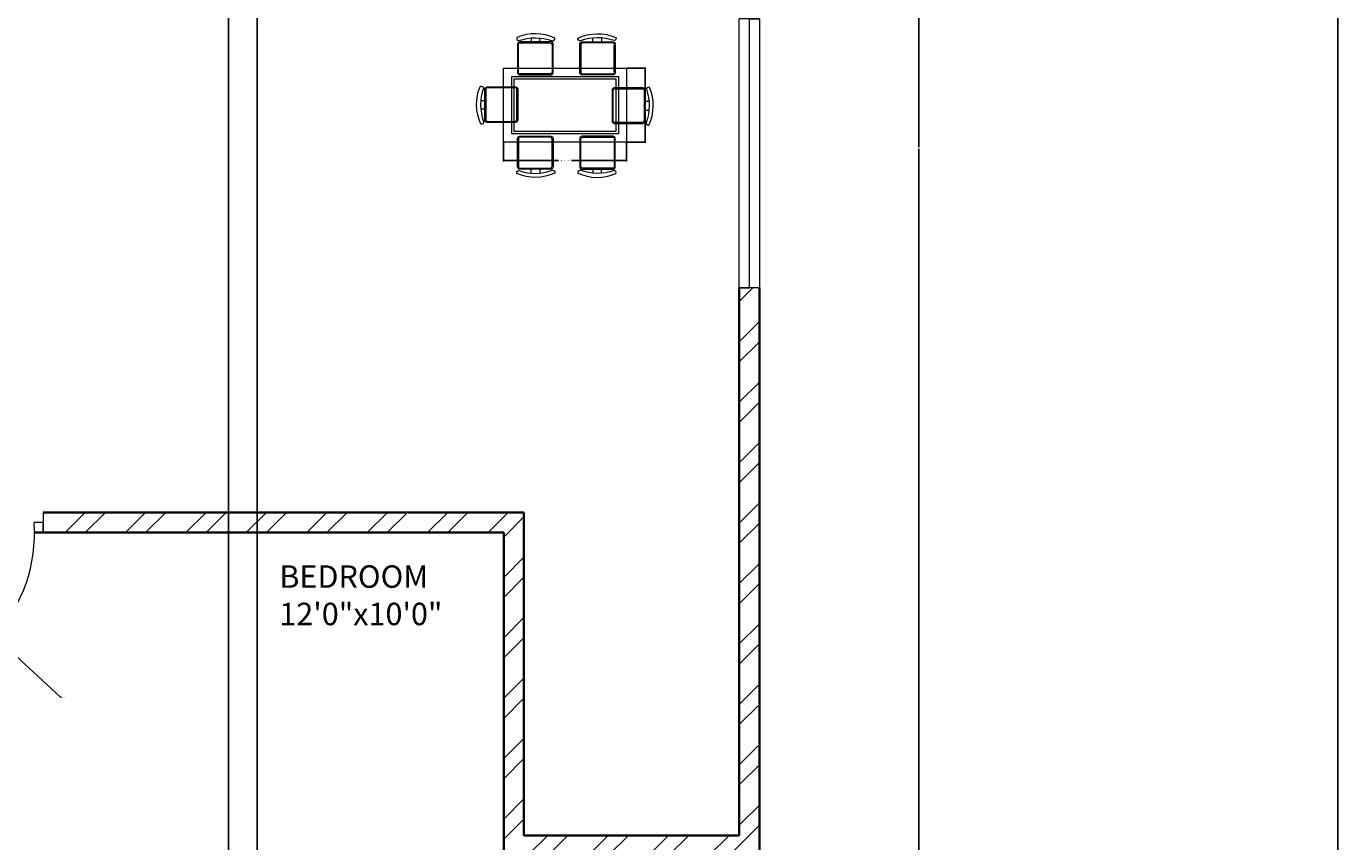
# Model space of a CAD drawing. Units: inches. Extents: x 2064 to 2782, y 1196 to 2299.
# Tile 10 of 11: x 2490 to 2782, y 1783 to 1965. Entities that reach past the tile are written whole.
import ezdxf

# ---------------------------------------------------------------- set-up
doc = ezdxf.new("R2010")
doc.units = ezdxf.units.IN
for name, color, linetype, lineweight in [('A-ANNO-DIMS', 2, 'Continuous', 18), ('A-ANNO-TTLB', 7, 'Continuous', 25), ('A-AREA-IDEN', 7, 'Continuous', 18), ('A-DOOR', 11, 'Continuous', 18), ('A-FURN', 8, 'Continuous', 13), ('A-GLAZ', 151, 'Continuous', 18), ('A-WALL', 7, 'Continuous', 35), ('A-WALL-PATT', 9, 'Continuous', 13)]:
    doc.layers.add(name, color=color, linetype=linetype, lineweight=lineweight)
doc.styles.get("Standard").update_dxf_attribs({"font": 'arial.ttf'})
doc.dimstyles.get("Standard").update_dxf_attribs({"dimtxt": 0.18, "dimasz": 0.18, "dimexe": 0.18, "dimexo": 0.0625, "dimgap": 0.09, "dimtad": 0, "dimtih": 1, "dimtoh": 1, "dimdec": 4, "dimzin": 0, "dimdsep": 46, "dimtxsty": 'Standard', "dimcen": 0.09, "dimadec": 0, "dimazin": 0, "dimtfac": 1, "dimtdec": 4, "dimtofl": 0, "dimtmove": 0, "dimatfit": 3, "dimfxl": 1, "dimtolj": 1, "dimtzin": 0, "dimarcsym": 0})

# ---------------------------------------------------------------- blocks, each defined once
blk = doc.blocks.new('WIN-60IN')
for p, q in [((0, 4.5), (0, 0)), ((60, 4.5), (0, 4.5)), ((60, 2.25), (60, 4.5)), ((60, 4.5), (60, 0)), ((0, 0), (0, 2.25)), ((0, 2.25), (60, 2.25)), ((0, 0), (60, 0))]:
    blk.add_line(p, q)
blk = doc.blocks.new('TABLE-DINING')
for points in [[(0, 16.47), (27.45, 16.47), (27.45, 0), (0, 0)], [(0, 16.47), (27.45, 16.47), (27.45, 0), (0, 0)], [(1.83, 14.64), (25.62, 14.64), (25.62, 1.83), (1.83, 1.83)], [(1.83, 14.64), (25.62, 14.64), (25.62, 1.83), (1.83, 1.83)], [(2.38, 14.09), (25.07, 14.09), (25.07, 2.38), (2.38, 2.38)], [(2.38, 14.09), (25.07, 14.09), (25.07, 2.38), (2.38, 2.38)]]:
    blk.add_lwpolyline(points, close=True)
blk = doc.blocks.new('*D16')
at = {"layer": 'A-ANNO-DIMS', "color": 0, "lineweight": -2, "transparency": 16777216}
for p, q in [((2596.11, 1938.78), (2596.11, 1934.54)), ((2623.56, 1938.78), (2623.56, 1934.54)), ((2596.29, 1934.72), (2608.4, 1934.72)), ((2623.38, 1934.72), (2611.27, 1934.72))]:
    blk.add_line(p, q, dxfattribs=at)
at = {"layer": 'A-ANNO-DIMS', "color": 0, "transparency": 16777216}
for points in [[(2596.29, 1934.75), (2596.29, 1934.69), (2596.11, 1934.72)], [(2623.38, 1934.75), (2623.38, 1934.69), (2623.56, 1934.72)]]:
    blk.add_solid(points, dxfattribs=at)
at = {"layer": 'Defpoints', "color": 0, "transparency": 16777216}
for p in [(2596.11, 1938.84), (2623.56, 1938.84), (2623.56, 1934.72)]:
    blk.add_point(p, dxfattribs=at)
at = {"layer": 'A-ANNO-DIMS', "color": 0, "transparency": 16777216, "insert": (2609.84, 1934.72), "char_height": 0.18, "attachment_point": 5}
blk.add_mtext('\\A1;DINING TABLE 27 TYP.', dxfattribs=at)
blk = doc.blocks.new('*D17')
at = {"layer": 'A-ANNO-DIMS', "color": 0, "lineweight": -2, "transparency": 16777216}
for p, q in [((2623.62, 1955.31), (2627.85, 1955.31)), ((2627.67, 1955.13), (2627.67, 1947.25)), ((2627.67, 1939.02), (2627.67, 1946.89)), ((2623.62, 1938.84), (2627.85, 1938.84))]:
    blk.add_line(p, q, dxfattribs=at)
at = {"layer": 'A-ANNO-DIMS', "color": 0, "transparency": 16777216}
for points in [[(2627.64, 1955.13), (2627.7, 1955.13), (2627.67, 1955.31)], [(2627.64, 1939.02), (2627.7, 1939.02), (2627.67, 1938.84)]]:
    blk.add_solid(points, dxfattribs=at)
at = {"layer": 'Defpoints', "color": 0, "transparency": 16777216}
for p in [(2623.56, 1955.31), (2627.67, 1955.31), (2623.56, 1938.84)]:
    blk.add_point(p, dxfattribs=at)
at = {"layer": 'A-ANNO-DIMS', "color": 0, "transparency": 16777216, "insert": (2627.67, 1947.07), "char_height": 0.18, "attachment_point": 5}
blk.add_mtext('\\A1;16 TYP.', dxfattribs=at)
blk = doc.blocks.new('*D23')
at = {"layer": 'A-ANNO-DIMS', "color": 0, "lineweight": -2, "transparency": 16777216}
for p, q in [((2653.23, 2234.29), (2688.85, 2234.29)), ((2688.67, 2234.11), (2688.67, 1937.72)), ((2688.67, 1640.97), (2688.67, 1937.36)), ((2452.23, 1640.79), (2688.85, 1640.79))]:
    blk.add_line(p, q, dxfattribs=at)
at = {"layer": 'A-ANNO-DIMS', "color": 0, "transparency": 16777216}
for points in [[(2688.64, 2234.11), (2688.7, 2234.11), (2688.67, 2234.29)], [(2688.64, 1640.97), (2688.7, 1640.97), (2688.67, 1640.79)]]:
    blk.add_solid(points, dxfattribs=at)
at = {"layer": 'Defpoints', "color": 0, "transparency": 16777216}
for p in [(2653.17, 2234.29), (2688.67, 2234.29), (2452.17, 1640.79)]:
    blk.add_point(p, dxfattribs=at)
at = {"layer": 'A-ANNO-DIMS', "color": 0, "transparency": 16777216, "insert": (2688.67, 1937.54), "char_height": 0.18, "attachment_point": 5}
blk.add_mtext('\\A1;593.5', dxfattribs=at)
blk = doc.blocks.new('*D27')
at = {"layer": 'A-ANNO-DIMS', "color": 0, "lineweight": -2, "transparency": 16777216}
for p, q in [((2452.17, 1640.85), (2452.17, 2269.97)), ((2452.35, 2269.79), (2493.09, 2269.79)), ((2534.61, 2269.79), (2493.87, 2269.79)), ((2534.79, 1643.35), (2534.79, 2269.97))]:
    blk.add_line(p, q, dxfattribs=at)
at = {"layer": 'A-ANNO-DIMS', "color": 0, "transparency": 16777216}
for points in [[(2452.35, 2269.82), (2452.35, 2269.76), (2452.17, 2269.79)], [(2534.61, 2269.82), (2534.61, 2269.76), (2534.79, 2269.79)]]:
    blk.add_solid(points, dxfattribs=at)
at = {"layer": 'Defpoints', "color": 0, "transparency": 16777216}
for p in [(2534.79, 2269.79), (2534.79, 1643.29), (2452.17, 1640.79)]:
    blk.add_point(p, dxfattribs=at)
at = {"layer": 'A-ANNO-DIMS', "color": 0, "transparency": 16777216, "insert": (2493.48, 2269.79), "char_height": 0.18, "attachment_point": 5}
blk.add_mtext('\\A1;82.62', dxfattribs=at)
blk = doc.blocks.new('*D36')
at = {"layer": 'A-ANNO-DIMS', "color": 0, "lineweight": -2, "transparency": 16777216}
for p, q in [((2390.62, 2058.73), (2390.62, 1539.01)), ((2541.17, 2058.73), (2541.17, 1539.01)), ((2390.8, 1539.19), (2465.44, 1539.19)), ((2540.99, 1539.19), (2466.35, 1539.19))]:
    blk.add_line(p, q, dxfattribs=at)
at = {"layer": 'A-ANNO-DIMS', "color": 0, "transparency": 16777216}
for points in [[(2390.8, 1539.22), (2390.8, 1539.16), (2390.62, 1539.19)], [(2540.99, 1539.22), (2540.99, 1539.16), (2541.17, 1539.19)]]:
    blk.add_solid(points, dxfattribs=at)
at = {"layer": 'Defpoints', "color": 0, "transparency": 16777216}
for p in [(2390.62, 2058.79), (2541.17, 2058.79), (2541.17, 1539.19)]:
    blk.add_point(p, dxfattribs=at)
at = {"layer": 'A-ANNO-DIMS', "color": 0, "transparency": 16777216, "insert": (2465.9, 1539.19), "char_height": 0.18, "attachment_point": 5}
blk.add_mtext('\\A1;150.55', dxfattribs=at)
blk = doc.blocks.new('*D42')
at = {"layer": 'A-ANNO-DIMS', "color": 0, "lineweight": -2, "transparency": 16777216}
for p, q in [((2457.99, 1851.52), (2458.17, 1851.52)), ((2458.08, 1851.43), (2458.08, 1851.61)), ((2497.35, 1815.1), (2482.76, 1828.63)), ((2497.53, 1815.1), (2497.35, 1815.1))]:
    blk.add_line(p, q, dxfattribs=at)
at = {"layer": 'A-ANNO-DIMS', "color": 0, "transparency": 16777216}
blk.add_solid([(2482.78, 1828.66), (2482.74, 1828.61), (2482.63, 1828.76)], dxfattribs=at)
at = {"layer": 'Defpoints', "color": 0, "transparency": 16777216}
for p in [(2458.08, 1851.52), (2482.63, 1828.76)]:
    blk.add_point(p, dxfattribs=at)
at = {"layer": 'A-ANNO-DIMS', "color": 0, "transparency": 16777216, "insert": (2498.01, 1815.1), "char_height": 0.18, "attachment_point": 5}
blk.add_mtext('\\A1;R33.48', dxfattribs=at)

msp = doc.modelspace()

# ---------------------------------------------------------------- hatches: boundary and pattern name
at = {"layer": 'A-WALL-PATT'}
h = msp.add_hatch(dxfattribs=at)
h.set_pattern_fill('ANSI32', color=256)
h.paths.add_polyline_path([(2489.7688, 2189.2917), (2574.5454, 2189.2917), (2574.5454, 2191.5417), (2574.5454, 2193.7917), (2570.6691, 2193.7917), (2570.6691, 2197.3052), (2568.4191, 2197.3052), (2566.1691, 2197.3052), (2566.1691, 2193.7917), (2494.1691, 2193.7917), (2494.1691, 2229.7917), (2523.2441, 2229.7917), (2523.2441, 2234.2917), (2471.2886, 2234.2917), (2471.2886, 2229.7917), (2489.6691, 2229.7917), (2489.6691, 2193.7917), (2417.6691, 2193.7917), (2417.6691, 2197.0632), (2415.4191, 2197.0632), (2413.1691, 2197.0632), (2413.1691, 2193.7917), (2406.8865, 2193.7917), (2406.8865, 2189.2917), (2485.2688, 2189.2917), (2485.2688, 2063.2917), (2369.1629, 2063.2917), (2369.1629, 2058.7917), (2386.1222, 2058.7917), (2386.1222, 1856.2917), (2382.1576, 1856.2917), (2382.1576, 1851.7917), (2394.9764, 1851.7917), (2394.9764, 1854.0417), (2394.9764, 1856.2917), (2390.6222, 1856.2917), (2390.6222, 2058.7917), (2485.2688, 2058.7917), (2493.762, 2058.7917), (2493.762, 2061.0417), (2493.762, 2063.2917), (2489.7688, 2063.2917)])
h.paths.add_polyline_path([(2447.2886, 2234.2917), (2413.1691, 2234.2917), (2413.1691, 2217.3799), (2417.6691, 2217.3799), (2417.6691, 2229.7917), (2447.2886, 2229.7917)], flags=17)
h.paths.add_polyline_path([(2570.6691, 2234.2917), (2547.2441, 2234.2917), (2547.2441, 2229.7917), (2566.1691, 2229.7917), (2566.1691, 2216.5615), (2570.6691, 2216.5615)], flags=17)
h.paths.add_polyline_path([(2653.1691, 2189.2917), (2653.1691, 2193.7917), (2640.8843, 2193.7917), (2640.8843, 2189.2917), (2648.6691, 2189.2917), (2648.6691, 2162.7138), (2653.1691, 2162.7138)])
h.paths.add_polyline_path([(2653.1691, 2102.7138), (2648.6691, 2102.7138), (2648.6691, 2063.2917), (2526.7281, 2063.2917), (2526.7281, 2058.7917), (2541.1691, 2058.7917), (2541.1691, 1993.2917), (2545.6691, 1993.2917), (2545.6691, 1997.7917), (2545.6691, 2058.7917), (2648.6691, 2058.7917), (2648.6691, 2050.1099), (2653.1691, 2050.1099)])
h.paths.add_polyline_path([(2600.6691, 1856.2917), (2493.4607, 1856.2917), (2493.4607, 1851.7917), (2596.1691, 1851.7917), (2596.1691, 1695.7917), (2594.0816, 1695.7917), (2594.0816, 1691.2917), (2614.7905, 1691.2917), (2614.7905, 1645.2917), (2536.7905, 1645.2917), (2536.7905, 1691.2917), (2539.332, 1691.2917), (2539.332, 1693.5417), (2539.332, 1695.7917), (2452.1691, 1695.7917), (2452.1691, 1851.7917), (2456.0775, 1851.7917), (2456.0775, 1856.2917), (2427.1536, 1856.2917), (2427.1536, 1851.7917), (2447.6691, 1851.7917), (2447.6691, 1695.7917), (2447.6691, 1645.2917), (2405.1469, 1645.2917), (2405.1469, 1640.7917), (2452.1691, 1640.7917), (2452.1691, 1645.2917), (2452.1691, 1691.2917), (2534.7905, 1691.2917), (2534.7905, 1645.2917), (2534.7905, 1643.2917), (2614.7905, 1643.2917), (2616.7905, 1643.2917), (2616.7905, 1691.2917), (2622.4029, 1691.2917), (2622.4029, 1693.7143), (2622.4029, 1695.7917), (2600.6691, 1695.7917), (2600.6691, 1779.7917), (2648.6691, 1779.7917), (2648.6691, 1695.7917), (2646.4029, 1695.7917), (2646.4029, 1691.2917), (2653.1691, 1691.2917), (2653.1691, 1906.3508), (2648.6691, 1906.3508), (2648.6691, 1856.2917), (2648.6691, 1784.2917), (2600.6691, 1784.2917)])
h.paths.add_polyline_path([(2322.9532, 1819.5181), (2320.7032, 1819.5181), (2318.4532, 1819.5181), (2318.4532, 1695.7917), (2242.7664, 1695.7917), (2242.7664, 1691.2917), (2318.4532, 1691.2917), (2318.4532, 1640.7917), (2322.9532, 1640.7917), (2345.1469, 1640.7917), (2345.1469, 1643.0417), (2345.1469, 1645.2917), (2322.9532, 1645.2917), (2322.9532, 1691.2917), (2322.9532, 1695.7917)])
h.paths.add_polyline_path([(2166.1825, 1691.2917), (2164.1825, 1691.2917), (2164.1825, 1643.2917), (2166.1825, 1643.2917), (2246.1825, 1643.2917), (2246.1825, 1645.2917), (2246.1825, 1691.2917), (2244.1825, 1691.2917), (2244.1825, 1645.2917), (2166.1825, 1645.2917)])
h.paths.add_polyline_path([(2309.404, 1932.7917), (2204.1691, 1932.7917), (2204.1691, 1960.0962), (2199.6691, 1960.0962), (2199.6691, 1932.7917), (2132.6691, 1932.7917), (2132.6691, 1951.0737), (2128.1691, 1951.0737), (2128.1691, 1910.0412), (2132.6691, 1910.0412), (2132.6691, 1928.2917), (2304.904, 1928.2917), (2304.904, 1856.2917), (2304.904, 1851.7917), (2318.4532, 1851.7917), (2318.4532, 1848.8308), (2322.9532, 1848.8308), (2322.9532, 1851.7917), (2347.7631, 1851.7917), (2347.7631, 1856.2917), (2309.404, 1856.2917)])
h.paths.add_polyline_path([(2132.6691, 2044.9092), (2130.4191, 2044.9092), (2128.1691, 2044.9092), (2128.1691, 1987.0737), (2132.6691, 1987.0737), (2132.6691, 2004.7917), (2199.6691, 2004.7917), (2204.1691, 2004.7917), (2204.1691, 2009.2917), (2132.6691, 2009.2917)])
h.paths.add_polyline_path([(2186.6691, 2195.9329), (2184.4191, 2195.9329), (2184.4191, 2195.8929), (2182.1691, 2195.9329), (2182.1691, 2193.7917), (2128.1691, 2193.7917), (2128.1691, 2181.4967), (2132.6691, 2181.4967), (2132.6691, 2182.7769), (2132.6691, 2189.2917), (2182.1691, 2189.2917), (2182.1691, 2135.2917), (2179.804, 2135.2917), (2179.804, 2130.7917), (2190.215, 2130.7917), (2190.215, 2133.0417), (2190.215, 2135.2917), (2186.6691, 2135.2917)])
h.paths.add_polyline_path([(2340.0628, 2189.2917), (2340.0628, 2191.5417), (2340.0628, 2193.7917), (2335.1691, 2193.7917), (2335.1691, 2234.2917), (2280.6746, 2234.2917), (2280.6746, 2229.7917), (2330.6691, 2229.7917), (2330.6691, 2193.7917), (2330.6691, 2135.2917), (2218.6309, 2135.2917), (2218.6309, 2130.7917), (2330.7688, 2130.7917), (2330.7688, 2008.4023), (2335.2688, 2008.4023), (2335.2688, 2058.7917), (2338.9208, 2058.7917), (2338.9208, 2061.0417), (2338.9208, 2063.2917), (2335.2688, 2063.2917), (2335.2688, 2189.2917)])
h.paths.add_polyline_path([(2220.6746, 2234.2917), (2182.1691, 2234.2917), (2182.1691, 2227.4187), (2186.6691, 2227.4187), (2186.6691, 2229.7917), (2220.6746, 2229.7917), (2220.6746, 2232.0417)])
h.paths.add_polyline_path([(2158.8146, 2135.2917), (2132.6691, 2135.2917), (2132.6691, 2157.4967), (2128.1691, 2157.4967), (2128.1691, 2104.9092), (2132.6691, 2104.9092), (2132.6691, 2130.7917), (2158.8146, 2130.7917), (2158.8146, 2133.0417)])
h.paths.add_polyline_path([(2396.0464, 2062.2045), (2434.8868, 2062.2045), (2434.8868, 2080.8619), (2396.0464, 2080.8619)], flags=24)
h.paths.add_polyline_path([(2196.1396, 1653.3449), (2232.023, 1653.3449), (2232.023, 1672.0022), (2196.1396, 1672.0022)], flags=25)

# ---------------------------------------------------------------- linework, layer by layer
at = {"layer": 'A-ANNO-TTLB'}
msp.add_lwpolyline([(2063.9994, 2298.574), (2782.0941, 2298.574), (2782.0941, 1490.6238), (2063.9994, 1490.6238)], close=True, dxfattribs=at)
at = {"layer": 'A-DOOR'}
for p, q in [((2493.4607, 1854.0417), (2491.4607, 1854.0417)), ((2493.4607, 1856.2917), (2493.4607, 1851.7917)), ((2493.4607, 1851.7917), (2493.4607, 1854.0417))]:
    msp.add_line(p, q, dxfattribs=at)
msp.add_arc((2458.0775, 1851.5199), 33.4783, 270, 4.319874, dxfattribs=at)
at = {"layer": 'A-FURN'}
for points in [[(2599.5069, 1961.4664, -0.17580919), (2606.9824, 1961.4098, 0.57839206), (2607.5487, 1962.0325, 0.21452438), (2599.1105, 1962.1457, 0.55201397), (2599.5069, 1961.4664, -0.06507904)], [(2599.507, 1961.4661, -0.17580919), (2606.9824, 1961.4095, 0.57839206), (2607.5487, 1962.0322, 0.21452438), (2599.1105, 1962.1454, 0.55201397), (2599.507, 1961.4661, -0.06507904)], [(2604.2276, 1961.1664), (2604.2276, 1962.0441, -0.06475861)], [(2604.2276, 1961.1661), (2604.2276, 1962.0438, -0.06475861)], [(2613.2757, 1961.4098, -0.57839206), (2612.7094, 1962.0325, -0.21452438), (2621.1476, 1962.1457, -0.55201397), (2620.7512, 1961.4664, 0.1758092), (2613.2757, 1961.4098)], [(2613.2757, 1961.4095, -0.57839206), (2612.7094, 1962.0322, -0.21452438), (2621.1476, 1962.1454, -0.55201397), (2620.7512, 1961.4661, 0.1758092), (2613.2758, 1961.4095)], [(2616.0305, 1961.1664), (2616.0305, 1962.0441, 0.06475861)], [(2616.0306, 1961.1661), (2616.0306, 1962.0438, 0.06475861)], [(2606.6652, 1961.1664), (2599.7253, 1961.1664, 0.41421356), (2599.2398, 1960.6809), (2599.2398, 1954.2997, 0.41421356), (2599.7253, 1953.8142), (2606.6652, 1953.8142, 0.41421356), (2607.1508, 1954.2997), (2607.1508, 1960.6809, 0.41421356), (2606.6652, 1961.1664)], [(2606.6652, 1961.1661), (2599.7253, 1961.1661, 0.41421356), (2599.2398, 1960.6806), (2599.2398, 1954.2994, 0.41421356), (2599.7253, 1953.8139), (2606.6652, 1953.8139, 0.41421356), (2607.1508, 1954.2994), (2607.1508, 1960.6806, 0.41421356), (2606.6652, 1961.1661)], [(2620.5328, 1961.1664, -0.41421356), (2621.0184, 1960.6809), (2621.0184, 1954.2997, -0.41421356), (2620.5328, 1953.8142), (2613.5929, 1953.8142, -0.41421356), (2613.1074, 1954.2997), (2613.1074, 1960.6809, -0.41421356), (2613.5929, 1961.1664), (2620.5328, 1961.1664)], [(2620.5328, 1961.1661, -0.41421356), (2621.0184, 1960.6806), (2621.0184, 1954.2994, -0.41421356), (2620.5328, 1953.8139), (2613.5929, 1953.8139, -0.41421356), (2613.1074, 1954.2994), (2613.1074, 1960.6806, -0.41421356), (2613.5929, 1961.1661), (2620.5328, 1961.1661)], [(2591.6862, 1943.4144, -0.57839206), (2591.0635, 1942.848, -0.21452438), (2590.9503, 1951.2862, -0.55201397), (2591.6296, 1950.8898, 0.17580937), (2591.6862, 1943.4144)], [(2591.6862, 1943.4141, -0.57839206), (2591.0635, 1942.8478, -0.21452438), (2590.9503, 1951.2859, -0.55201397), (2591.6296, 1950.8895, 0.17580937), (2591.6862, 1943.4141)], [(2591.9296, 1950.6715, -0.41421356), (2592.4151, 1951.157), (2598.7963, 1951.157, -0.41421356), (2599.2818, 1950.6715), (2599.2818, 1943.7315, -0.41421356), (2598.7963, 1943.246), (2592.4151, 1943.246, -0.41421356), (2591.9296, 1943.7315), (2591.9296, 1950.6715)], [(2591.9296, 1950.6712, -0.41421356), (2592.4152, 1951.1567), (2598.7963, 1951.1567, -0.41421356), (2599.2818, 1950.6712), (2599.2818, 1943.7312, -0.41421356), (2598.7963, 1943.2457), (2592.4152, 1943.2457, -0.41421356), (2591.9296, 1943.7312), (2591.9296, 1950.6712)], [(2627.6671, 1950.4338, 0.41421356), (2627.1816, 1950.9193), (2620.8004, 1950.9193, 0.41421356), (2620.3149, 1950.4338), (2620.3149, 1943.4938, 0.41421356), (2620.8004, 1943.0083), (2627.1816, 1943.0083, 0.41421356), (2627.6671, 1943.4938), (2627.6671, 1950.4338)], [(2627.6671, 1950.4335, 0.41421356), (2627.1816, 1950.919), (2620.8004, 1950.919, 0.41421356), (2620.3149, 1950.4335), (2620.3149, 1943.4935, 0.41421356), (2620.8004, 1943.008), (2627.1816, 1943.008, 0.41421356), (2627.6671, 1943.4935), (2627.6671, 1950.4335)], [(2627.9671, 1950.6521, -0.17580919), (2627.9105, 1943.1767, 0.57839206), (2628.5332, 1942.6104, 0.21452438), (2628.6464, 1951.0485, 0.55201397), (2627.9671, 1950.6521, -0.06507904)], [(2627.9671, 1950.6518, -0.17580919), (2627.9105, 1943.1764, 0.57839206), (2628.5332, 1942.6101, 0.21452438), (2628.6464, 1951.0483, 0.55201397), (2627.9671, 1950.6518, -0.06507904)], [(2591.9296, 1946.1692), (2591.0519, 1946.1692, 0.06475861)], [(2591.9296, 1946.1689), (2591.0519, 1946.1689, 0.06475861)], [(2627.6671, 1945.9315), (2628.5448, 1945.9315, -0.06475861)], [(2627.6671, 1945.9312), (2628.5448, 1945.9312, -0.06475861)], [(2606.6652, 1932.8006), (2599.7253, 1932.8006, -0.41421356), (2599.2398, 1933.2862), (2599.2398, 1939.6673, -0.41421356), (2599.7253, 1940.1528), (2606.6652, 1940.1528, -0.41421356), (2607.1508, 1939.6673), (2607.1508, 1933.2862, -0.41421356), (2606.6652, 1932.8006)], [(2606.6652, 1932.8003), (2599.7253, 1932.8003, -0.41421356), (2599.2398, 1933.2859), (2599.2398, 1939.667, -0.41421356), (2599.7253, 1940.1525), (2606.6652, 1940.1525, -0.41421356), (2607.1508, 1939.667), (2607.1508, 1933.2859, -0.41421356), (2606.6652, 1932.8003)], [(2620.5328, 1932.8006, 0.41421356), (2621.0184, 1933.2862), (2621.0184, 1939.6673, 0.41421356), (2620.5328, 1940.1528), (2613.5929, 1940.1528, 0.41421356), (2613.1074, 1939.6673), (2613.1074, 1933.2862, 0.41421356), (2613.5929, 1932.8006), (2620.5328, 1932.8006)], [(2620.5328, 1932.8003, 0.41421356), (2621.0184, 1933.2859), (2621.0184, 1939.667, 0.41421356), (2620.5328, 1940.1525), (2613.5929, 1940.1525, 0.41421356), (2613.1074, 1939.667), (2613.1074, 1933.2859, 0.41421356), (2613.5929, 1932.8003), (2620.5328, 1932.8003)], [(2604.2276, 1932.8006), (2604.2276, 1931.9229, 0.06475861)], [(2604.2276, 1932.8003), (2604.2276, 1931.9227, 0.06475861)], [(2616.0305, 1932.8006), (2616.0305, 1931.9229, -0.06475861)], [(2616.0306, 1932.8003), (2616.0306, 1931.9227, -0.06475861)], [(2606.9824, 1932.5572, -0.57839206), (2607.5487, 1931.9345, -0.21452438), (2599.1105, 1931.8213, -0.55201397), (2599.5069, 1932.5006, 0.17580929), (2606.9824, 1932.5572)], [(2606.9824, 1932.5569, -0.57839206), (2607.5487, 1931.9342, -0.21452438), (2599.1105, 1931.821, -0.55201397), (2599.507, 1932.5003, 0.17580929), (2606.9824, 1932.5569)], [(2620.7512, 1932.5006, -0.17580928), (2613.2757, 1932.5572, 0.57839206), (2612.7094, 1931.9345, 0.21452438), (2621.1476, 1931.8213, 0.55201397), (2620.7512, 1932.5006, -0.06507904)], [(2620.7512, 1932.5003, -0.17580928), (2613.2757, 1932.5569, 0.57839206), (2612.7094, 1931.9342, 0.21452438), (2621.1476, 1931.821, 0.55201397), (2620.7512, 1932.5003, -0.06507904)]]:
    msp.add_lwpolyline(points, format="xyb", dxfattribs=at)
for points in [[(2602.285, 1962.06), (2602.285, 1961.1664)], [(2602.285, 1962.0597), (2602.285, 1961.1661)], [(2617.9731, 1962.06), (2617.9731, 1961.1664)], [(2617.9731, 1962.0597), (2617.9731, 1961.1661)], [(2591.036, 1948.1118), (2591.9296, 1948.1118)], [(2591.036, 1948.1115), (2591.9296, 1948.1115)], [(2628.5607, 1947.8741), (2627.6671, 1947.8741)], [(2628.5607, 1947.8738), (2627.6671, 1947.8738)], [(2602.285, 1931.907), (2602.285, 1932.8006)], [(2602.285, 1931.9067), (2602.285, 1932.8003)], [(2617.9731, 1931.907), (2617.9731, 1932.8006)], [(2617.9731, 1931.9067), (2617.9731, 1932.8003)]]:
    msp.add_lwpolyline(points, dxfattribs=at)
for points in [[(2599.7282, 1960.9476), (2606.4465, 1960.9476, -0.41421356), (2606.932, 1960.4621), (2606.932, 1954.5184, -0.41421356), (2606.4465, 1954.0329), (2599.7282, 1954.0329, -0.51206948), (2599.4585, 1954.5184), (2599.4585, 1960.4621, -0.51206948)], [(2599.7282, 1960.9474), (2606.4465, 1960.9474, -0.41421356), (2606.932, 1960.4618), (2606.932, 1954.5182, -0.41421356), (2606.4465, 1954.0326), (2599.7282, 1954.0326, -0.51206948), (2599.4585, 1954.5182), (2599.4585, 1960.4618, -0.51206948)], [(2620.5299, 1960.9476), (2613.8116, 1960.9476, 0.41421356), (2613.3261, 1960.4621), (2613.3261, 1954.5184, 0.41421356), (2613.8116, 1954.0329), (2620.5299, 1954.0329, 0.51206948), (2620.7996, 1954.5184), (2620.7996, 1960.4621, 0.51206948)], [(2620.5299, 1960.9474), (2613.8116, 1960.9474, 0.41421356), (2613.3261, 1960.4618), (2613.3261, 1954.5182, 0.41421356), (2613.8116, 1954.0326), (2620.5299, 1954.0326, 0.51206948), (2620.7996, 1954.5182), (2620.7996, 1960.4618, 0.51206948)], [(2592.1483, 1950.6685), (2592.1483, 1943.9502, 0.41421356), (2592.6339, 1943.4647), (2598.5776, 1943.4647, 0.41421356), (2599.0631, 1943.9502), (2599.0631, 1950.6685, 0.51206948), (2598.5776, 1950.9382), (2592.6339, 1950.9382, 0.51206948)], [(2592.1484, 1950.6682), (2592.1484, 1943.95, 0.41421356), (2592.6339, 1943.4644), (2598.5776, 1943.4644, 0.41421356), (2599.0631, 1943.95), (2599.0631, 1950.6682, 0.51206948), (2598.5776, 1950.938), (2592.6339, 1950.938, 0.51206948)], [(2627.4483, 1950.4308), (2627.4483, 1943.7126, -0.41421356), (2626.9628, 1943.227), (2621.0191, 1943.227, -0.41421356), (2620.5336, 1943.7126), (2620.5336, 1950.4308, -0.51206948), (2621.0191, 1950.7006), (2626.9628, 1950.7006, -0.51206948)], [(2627.4484, 1950.4305), (2627.4484, 1943.7123, -0.41421356), (2626.9628, 1943.2268), (2621.0192, 1943.2268, -0.41421356), (2620.5336, 1943.7123), (2620.5336, 1950.4305, -0.51206948), (2621.0192, 1950.7003), (2626.9628, 1950.7003, -0.51206948)], [(2599.7282, 1933.0194), (2606.4465, 1933.0194, 0.41421356), (2606.932, 1933.5049), (2606.932, 1939.4486, 0.41421356), (2606.4465, 1939.9341), (2599.7282, 1939.9341, 0.51206948), (2599.4585, 1939.4486), (2599.4585, 1933.5049, 0.51206948)], [(2599.7282, 1933.0191), (2606.4465, 1933.0191, 0.41421356), (2606.932, 1933.5046), (2606.932, 1939.4483, 0.41421356), (2606.4465, 1939.9338), (2599.7282, 1939.9338, 0.51206948), (2599.4585, 1939.4483), (2599.4585, 1933.5046, 0.51206948)], [(2620.5299, 1933.0194), (2613.8116, 1933.0194, -0.41421356), (2613.3261, 1933.5049), (2613.3261, 1939.4486, -0.41421356), (2613.8116, 1939.9341), (2620.5299, 1939.9341, -0.51206948), (2620.7996, 1939.4486), (2620.7996, 1933.5049, -0.51206948)], [(2620.5299, 1933.0191), (2613.8116, 1933.0191, -0.41421356), (2613.3261, 1933.5046), (2613.3261, 1939.4483, -0.41421356), (2613.8116, 1939.9338), (2620.5299, 1939.9338, -0.51206948), (2620.7996, 1939.4483), (2620.7996, 1933.5046, -0.51206948)]]:
    msp.add_lwpolyline(points, format="xyb", close=True, dxfattribs=at)
at = {"layer": 'A-WALL'}
for p, q in [((2648.6691, 1856.2917), (2648.6691, 1906.3508)), ((2653.1691, 1906.3508), (2653.1691, 1691.2917)), ((2600.6691, 1856.2917), (2493.4607, 1856.2917)), ((2600.6691, 1784.2917), (2600.6691, 1856.2917)), ((2648.6691, 1784.2917), (2648.6691, 1856.2917)), ((2491.5547, 1851.7917), (2596.1691, 1851.7917)), ((2596.1691, 1695.7917), (2596.1691, 1851.7917)), ((2600.6691, 1784.2917), (2648.6691, 1784.2917))]:
    msp.add_line(p, q, dxfattribs=at)

# ---------------------------------------------------------------- block references
at = {"layer": 'A-FURN'}
msp.add_blockref('TABLE-DINING', (2596.1122, 1938.8377), dxfattribs=at)
at = {"layer": 'A-GLAZ', "extrusion": (0, 0, -1), "zscale": -1, "rotation": 90}
msp.add_blockref('WIN-60IN', (-2648.6691, 1906.3508), dxfattribs=at)

# ---------------------------------------------------------------- texts
at = {"layer": 'A-AREA-IDEN', "insert": (2546.1353, 1844.498), "char_height": 5, "attachment_point": 1}
msp.add_mtext_dynamic_manual_height_columns('BEDROOM\\P12\'0"x10\'0"', width=205.772299, gutter_width=12.5, heights=[0], dxfattribs=at)

# ---------------------------------------------------------------- dimensions: what is measured, and where the dimension line sits
at = {"layer": 'A-ANNO-DIMS'}
for base, p1, p2, picture, middle in [((2534.7905, 2269.7917), (2452.1691, 1640.7917), (2534.7905, 1643.2917), '*D27', (2493.4798, 2269.7917)), ((2541.1691, 1539.1896), (2390.6222, 2058.7917), (2541.1691, 2058.7917), '*D36', (2465.8957, 1539.1896))]:
    dim = msp.add_linear_dim(base=base, p1=p1, p2=p2, dimstyle='Standard', override={"dimdec": 2, "dimlfac": 1, "dimrnd": 0, "dimzin": 0, "dimdsep": 46, "dimlunit": 2}, dxfattribs=at)
    dim.commit()
    dim.dimension.update_dxf_attribs({"geometry": picture, "text_midpoint": middle})
dim = msp.add_linear_dim(base=(2688.6691, 2234.2917), p1=(2452.1691, 1640.7917), p2=(2653.1691, 2234.2917), angle=90, dimstyle='Standard', override={"dimdec": 1, "dimlfac": 1, "dimrnd": 0, "dimzin": 0, "dimdsep": 46, "dimlunit": 2}, dxfattribs=at)
dim.commit()
dim.dimension.update_dxf_attribs({"geometry": '*D23', "text_midpoint": (2688.6691, 1937.5417)})
dim = msp.add_linear_dim(base=(2627.6748, 1955.3054), p1=(2623.5579, 1938.8377), p2=(2623.5579, 1955.3054), angle=90, text='<> TYP.', dimstyle='Standard', override={"dimdec": 0, "dimlfac": 1, "dimrnd": 0, "dimzin": 0, "dimdsep": 46, "dimlunit": 2}, dxfattribs=at)
dim.commit()
dim.dimension.update_dxf_attribs({"geometry": '*D17', "text_midpoint": (2627.6748, 1947.0716)})
dim = msp.add_linear_dim(base=(2623.5579, 1934.7208), p1=(2596.1122, 1938.8377), p2=(2623.5579, 1938.8377), text='DINING TABLE <> TYP.', dimstyle='Standard', override={"dimdec": 0, "dimlfac": 1, "dimrnd": 0, "dimzin": 0, "dimdsep": 46, "dimlunit": 2}, dxfattribs=at)
dim.commit()
dim.dimension.update_dxf_attribs({"geometry": '*D16', "text_midpoint": (2609.8351, 1934.7208)})
dim = msp.add_radius_dim(center=(2458.0775, 1851.5199), mpoint=(2482.6257, 1828.7563), dimstyle='Standard', override={"dimdec": 2, "dimlfac": 1, "dimrnd": 0, "dimzin": 0, "dimdsep": 46, "dimlunit": 2}, dxfattribs=at)
dim.commit()
dim.dimension.update_dxf_attribs({"geometry": '*D42', "text_midpoint": (2498.0146, 1815.0982), "dimtype": 164})

doc.saveas('drawing.dxf')
